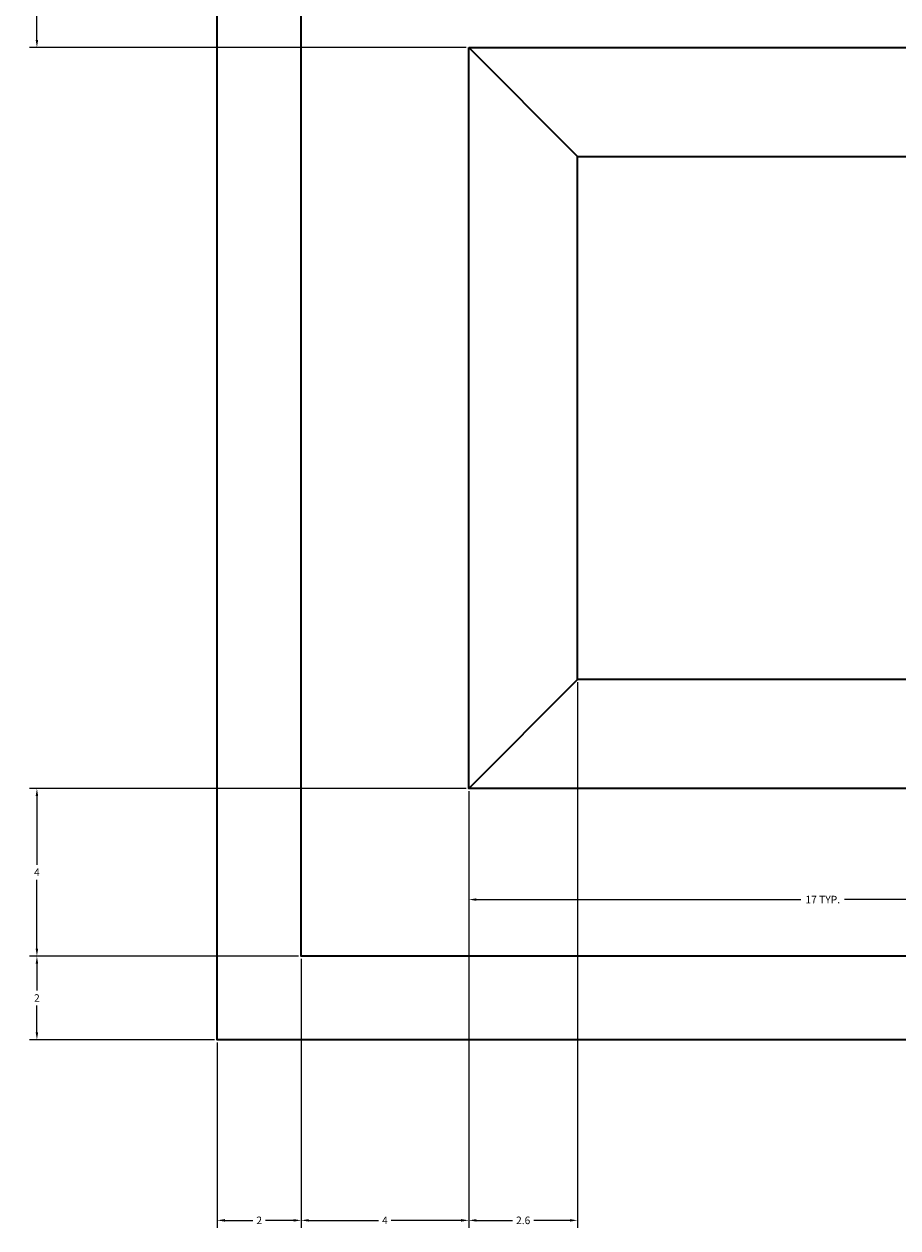
# Model space of a CAD drawing. Units: inches. Extents: x 3137 to 3299, y 1994 to 2089.
# Tile 8 of 14: x 3230 to 3251, y 1996 to 2024. Entities that reach past the tile are written whole.
import ezdxf

# ---------------------------------------------------------------- set-up
doc = ezdxf.new("R2010")
doc.units = ezdxf.units.IN
doc.header["$MEASUREMENT"] = 0
doc.layers.add('A-ANNO-DIMS', color=2, linetype='Continuous', lineweight=18)
doc.layers.add('A-DOOR', color=4, linetype='Continuous', lineweight=35)
doc.styles.get("Standard").update_dxf_attribs({"font": 'arial.ttf'})
doc.dimstyles.get("Standard").update_dxf_attribs({"dimtxt": 0.18, "dimasz": 0.18, "dimexe": 0.18, "dimexo": 0.0625, "dimgap": 0.09, "dimtad": 0, "dimtih": 1, "dimtoh": 1, "dimdec": 4, "dimzin": 0, "dimdsep": 46, "dimtxsty": 'Standard', "dimcen": 0.09, "dimadec": 0, "dimazin": 0, "dimtfac": 1, "dimtdec": 4, "dimtofl": 0, "dimtmove": 0, "dimatfit": 3, "dimfxl": 1, "dimtolj": 1, "dimtzin": 0, "dimarcsym": 0})

# ---------------------------------------------------------------- blocks, each defined once
blk = doc.blocks.new('DOOR-PANEL-RAISED-BOT')
for p, q in [((0, 17.675), (16.9, 17.675)), ((2.6, 15.075), (0, 17.675)), ((14.3, 15.075), (16.9, 17.675)), ((16.9, 0), (16.9, 17.675)), ((2.6, 15.075), (14.3, 15.075)), ((14.3, 2.6), (14.3, 15.075)), ((2.6, 2.6), (0, 0)), ((14.3, 2.6), (16.9, 0))]:
    blk.add_line(p, q)
for points in [[(16.9, 0), (0, 0), (0, 17.675)], [(14.3, 2.6), (2.6, 2.6), (2.6, 15.075)]]:
    blk.add_lwpolyline(points)
blk = doc.blocks.new('*D10')
at = {"layer": 'A-ANNO-DIMS', "color": 0, "lineweight": -2, "transparency": 16777216}
for p, q in [((3240.504, 2006.113), (3240.504, 2003.344)), ((3257.404, 2006.113), (3257.404, 2003.344)), ((3240.684, 2003.524), (3248.434, 2003.524)), ((3257.224, 2003.524), (3249.474, 2003.524))]:
    blk.add_line(p, q, dxfattribs=at)
at = {"layer": 'A-ANNO-DIMS', "color": 0, "transparency": 16777216}
for points in [[(3240.684, 2003.554), (3240.684, 2003.494), (3240.504, 2003.524)], [(3257.224, 2003.554), (3257.224, 2003.494), (3257.404, 2003.524)]]:
    blk.add_solid(points, dxfattribs=at)
at = {"layer": 'Defpoints', "color": 0, "transparency": 16777216}
for p in [(3240.504, 2006.176), (3257.404, 2006.176), (3257.404, 2003.524)]:
    blk.add_point(p, dxfattribs=at)
at = {"layer": 'A-ANNO-DIMS', "color": 0, "transparency": 16777216, "insert": (3248.954, 2003.524), "char_height": 0.18, "attachment_point": 5}
blk.add_mtext('\\A1;17 TYP.', dxfattribs=at)
blk = doc.blocks.new('*D56')
at = {"layer": 'A-ANNO-DIMS', "color": 0, "lineweight": -2, "transparency": 16777216}
for p, q in [((3236.504, 2002.113), (3236.504, 1995.691)), ((3234.504, 2000.113), (3234.504, 1995.691)), ((3234.684, 1995.871), (3235.354, 1995.871)), ((3236.324, 1995.871), (3235.654, 1995.871))]:
    blk.add_line(p, q, dxfattribs=at)
at = {"layer": 'A-ANNO-DIMS', "color": 0, "transparency": 16777216}
for points in [[(3234.684, 1995.901), (3234.684, 1995.841), (3234.504, 1995.871)], [(3236.324, 1995.901), (3236.324, 1995.841), (3236.504, 1995.871)]]:
    blk.add_solid(points, dxfattribs=at)
at = {"layer": 'Defpoints', "color": 0, "transparency": 16777216}
for p in [(3236.504, 2002.176), (3234.504, 2000.176), (3236.504, 1995.871)]:
    blk.add_point(p, dxfattribs=at)
at = {"layer": 'A-ANNO-DIMS', "color": 0, "transparency": 16777216, "insert": (3235.504, 1995.871), "char_height": 0.18, "attachment_point": 5}
blk.add_mtext('\\A1;2', dxfattribs=at)
blk = doc.blocks.new('*D57')
at = {"layer": 'A-ANNO-DIMS', "color": 0, "lineweight": -2, "transparency": 16777216}
for p, q in [((3240.504, 2006.113), (3240.504, 1995.691)), ((3236.504, 2002.113), (3236.504, 1995.691)), ((3236.684, 1995.871), (3238.352, 1995.871)), ((3240.324, 1995.871), (3238.656, 1995.871))]:
    blk.add_line(p, q, dxfattribs=at)
at = {"layer": 'A-ANNO-DIMS', "color": 0, "transparency": 16777216}
for points in [[(3236.684, 1995.901), (3236.684, 1995.841), (3236.504, 1995.871)], [(3240.324, 1995.901), (3240.324, 1995.841), (3240.504, 1995.871)]]:
    blk.add_solid(points, dxfattribs=at)
at = {"layer": 'Defpoints', "color": 0, "transparency": 16777216}
for p in [(3240.504, 2006.176), (3236.504, 2002.176), (3240.504, 1995.871)]:
    blk.add_point(p, dxfattribs=at)
at = {"layer": 'A-ANNO-DIMS', "color": 0, "transparency": 16777216, "insert": (3238.504, 1995.871), "char_height": 0.18, "attachment_point": 5}
blk.add_mtext('\\A1;4', dxfattribs=at)
blk = doc.blocks.new('*D58')
at = {"layer": 'A-ANNO-DIMS', "color": 0, "lineweight": -2, "transparency": 16777216}
for p, q in [((3243.104, 2008.713), (3243.104, 1995.691)), ((3240.504, 2006.113), (3240.504, 1995.691)), ((3240.684, 1995.871), (3241.549, 1995.871)), ((3242.924, 1995.871), (3242.059, 1995.871))]:
    blk.add_line(p, q, dxfattribs=at)
at = {"layer": 'A-ANNO-DIMS', "color": 0, "transparency": 16777216}
for points in [[(3240.684, 1995.901), (3240.684, 1995.841), (3240.504, 1995.871)], [(3242.924, 1995.901), (3242.924, 1995.841), (3243.104, 1995.871)]]:
    blk.add_solid(points, dxfattribs=at)
at = {"layer": 'Defpoints', "color": 0, "transparency": 16777216}
for p in [(3243.104, 2008.776), (3240.504, 2006.176), (3243.104, 1995.871)]:
    blk.add_point(p, dxfattribs=at)
at = {"layer": 'A-ANNO-DIMS', "color": 0, "transparency": 16777216, "insert": (3241.804, 1995.871), "char_height": 0.18, "attachment_point": 5}
blk.add_mtext('\\A1;2.6', dxfattribs=at)
blk = doc.blocks.new('*D66')
at = {"layer": 'A-ANNO-DIMS', "color": 0, "lineweight": -2, "transparency": 16777216}
for p, q in [((3236.441, 2002.176), (3230.019, 2002.176)), ((3230.199, 2001.996), (3230.199, 2001.356)), ((3230.199, 2000.356), (3230.199, 2000.995)), ((3234.441, 2000.176), (3230.019, 2000.176))]:
    blk.add_line(p, q, dxfattribs=at)
at = {"layer": 'A-ANNO-DIMS', "color": 0, "transparency": 16777216}
for points in [[(3230.169, 2001.996), (3230.229, 2001.996), (3230.199, 2002.176)], [(3230.169, 2000.356), (3230.229, 2000.356), (3230.199, 2000.176)]]:
    blk.add_solid(points, dxfattribs=at)
at = {"layer": 'Defpoints', "color": 0, "transparency": 16777216}
for p in [(3230.199, 2002.176), (3236.504, 2002.176), (3234.504, 2000.176)]:
    blk.add_point(p, dxfattribs=at)
at = {"layer": 'A-ANNO-DIMS', "color": 0, "transparency": 16777216, "insert": (3230.199, 2001.176), "char_height": 0.18, "attachment_point": 5}
blk.add_mtext('\\A1;2', dxfattribs=at)
blk = doc.blocks.new('*D67')
at = {"layer": 'A-ANNO-DIMS', "color": 0, "lineweight": -2, "transparency": 16777216}
for p, q in [((3240.441433, 2006.175607), (3230.018933, 2006.175607)), ((3230.198933, 2005.995607), (3230.198933, 2004.355607)), ((3230.198933, 2002.355607), (3230.198933, 2003.995607)), ((3236.441433, 2002.175607), (3230.018933, 2002.175607))]:
    blk.add_line(p, q, dxfattribs=at)
at = {"layer": 'A-ANNO-DIMS', "color": 0, "transparency": 16777216}
for points in [[(3230.168933, 2005.995607), (3230.228933, 2005.995607), (3230.198933, 2006.175607)], [(3230.168933, 2002.355607), (3230.228933, 2002.355607), (3230.198933, 2002.175607)]]:
    blk.add_solid(points, dxfattribs=at)
at = {"layer": 'Defpoints', "color": 0, "transparency": 16777216}
for p in [(3230.198933, 2006.175607), (3240.503933, 2006.175607), (3236.503933, 2002.175607)]:
    blk.add_point(p, dxfattribs=at)
at = {"layer": 'A-ANNO-DIMS', "color": 0, "transparency": 16777216, "insert": (3230.198933, 2004.175607), "char_height": 0.18, "attachment_point": 5}
blk.add_mtext('\\A1;4', dxfattribs=at)
blk = doc.blocks.new('*D68')
at = {"layer": 'A-ANNO-DIMS', "color": 0, "lineweight": -2, "transparency": 16777216}
for p, q in [((3240.441, 2028.676), (3230.019, 2028.676)), ((3230.199, 2028.496), (3230.199, 2026.445)), ((3230.199, 2024.031), (3230.199, 2026.082)), ((3240.441, 2023.851), (3230.019, 2023.851))]:
    blk.add_line(p, q, dxfattribs=at)
at = {"layer": 'A-ANNO-DIMS', "color": 0, "transparency": 16777216}
for points in [[(3230.169, 2028.496), (3230.229, 2028.496), (3230.199, 2028.676)], [(3230.169, 2024.031), (3230.229, 2024.031), (3230.199, 2023.851)]]:
    blk.add_solid(points, dxfattribs=at)
at = {"layer": 'Defpoints', "color": 0, "transparency": 16777216}
for p in [(3230.199, 2028.676), (3240.504, 2028.676), (3240.504, 2023.851)]:
    blk.add_point(p, dxfattribs=at)
at = {"layer": 'A-ANNO-DIMS', "color": 0, "transparency": 16777216, "insert": (3230.199, 2026.264), "char_height": 0.18, "attachment_point": 5}
blk.add_mtext('\\A1;4.825', dxfattribs=at)

msp = doc.modelspace()

# ---------------------------------------------------------------- linework, layer by layer
at = {"layer": 'A-DOOR'}
for points in [[(3234.5039, 2084.1756), (3294.5039, 2084.1756), (3294.5039, 2000.1756), (3234.5039, 2000.1756)], [(3236.5039, 2082.1756), (3292.5039, 2082.1756), (3292.5039, 2002.1756), (3236.5039, 2002.1756)]]:
    msp.add_lwpolyline(points, close=True, dxfattribs=at)

# ---------------------------------------------------------------- block references
msp.add_blockref('DOOR-PANEL-RAISED-BOT', (3240.504, 2006.176), dxfattribs=at)

# ---------------------------------------------------------------- dimensions: what is measured, and where the dimension line sits
at = {"layer": 'A-ANNO-DIMS'}
for base, p1, p2, override, picture, middle in [((3230.1989, 2028.6759), (3240.5039, 2023.8512), (3240.5039, 2028.6759), {"dimdec": 3, "dimlfac": 1, "dimrnd": 0, "dimzin": 0, "dimdsep": 46, "dimlunit": 2}, '*D68', (3230.1989, 2026.2636)), ((3230.1989, 2006.1756), (3236.5039, 2002.1756), (3240.5039, 2006.1756), {"dimdec": 0, "dimlfac": 1, "dimrnd": 0, "dimzin": 0, "dimdsep": 46, "dimlunit": 2}, '*D67', (3230.1989, 2004.1756)), ((3230.1989, 2002.1756), (3234.5039, 2000.1756), (3236.5039, 2002.1756), {"dimdec": 0, "dimlfac": 1, "dimrnd": 0, "dimzin": 0, "dimdsep": 46, "dimlunit": 2}, '*D66', (3230.1989, 2001.1756))]:
    dim = msp.add_linear_dim(base=base, p1=p1, p2=p2, angle=90, dimstyle='Standard', override=override, dxfattribs=at)
    dim.commit()
    dim.dimension.update_dxf_attribs({"geometry": picture, "text_midpoint": middle})
for base, p1, p2, override, picture, middle in [((3243.1039, 1995.8706), (3240.5039, 2006.1756), (3243.1039, 2008.7756), {"dimdec": 1, "dimlfac": 1, "dimrnd": 0, "dimzin": 0, "dimdsep": 46, "dimlunit": 2}, '*D58', (3241.8039, 1995.8706)), ((3240.5039, 1995.8706), (3236.5039, 2002.1756), (3240.5039, 2006.1756), {"dimdec": 0, "dimlfac": 1, "dimrnd": 0, "dimzin": 0, "dimdsep": 46, "dimlunit": 2}, '*D57', (3238.5039, 1995.8706)), ((3236.5039, 1995.8706), (3234.5039, 2000.1756), (3236.5039, 2002.1756), {"dimdec": 0, "dimlfac": 1, "dimrnd": 0, "dimzin": 0, "dimdsep": 46, "dimlunit": 2}, '*D56', (3235.5039, 1995.8706))]:
    dim = msp.add_linear_dim(base=base, p1=p1, p2=p2, dimstyle='Standard', override=override, dxfattribs=at)
    dim.commit()
    dim.dimension.update_dxf_attribs({"geometry": picture, "text_midpoint": middle})
dim = msp.add_linear_dim(base=(3257.4039, 2003.5243), p1=(3240.5039, 2006.1756), p2=(3257.4039, 2006.1756), text='<> TYP.', dimstyle='Standard', override={"dimdec": 0, "dimrnd": 0, "dimzin": 0, "dimlunit": 2}, dxfattribs=at)
dim.commit()
dim.dimension.update_dxf_attribs({"geometry": '*D10', "text_midpoint": (3248.9539, 2003.5243)})

doc.saveas('drawing.dxf')
